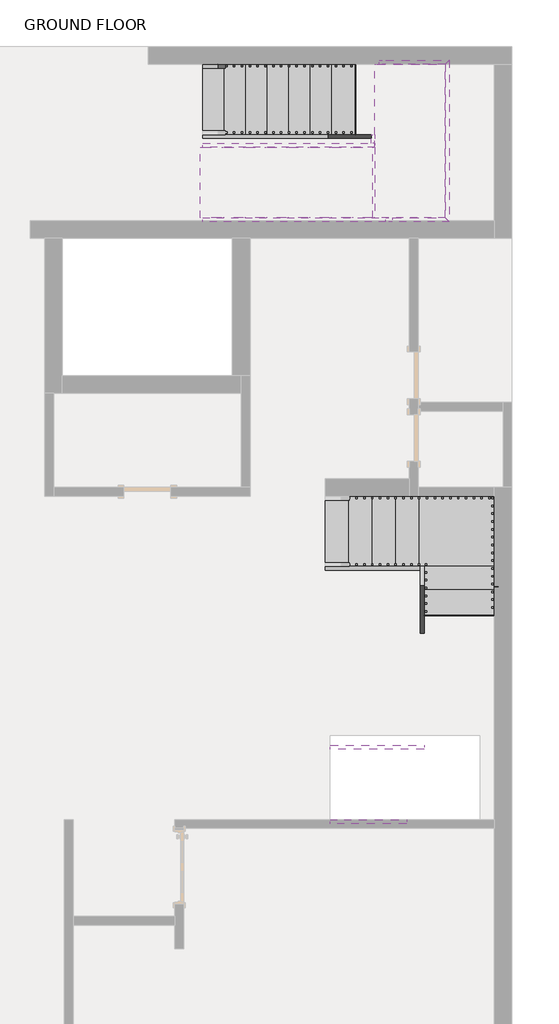
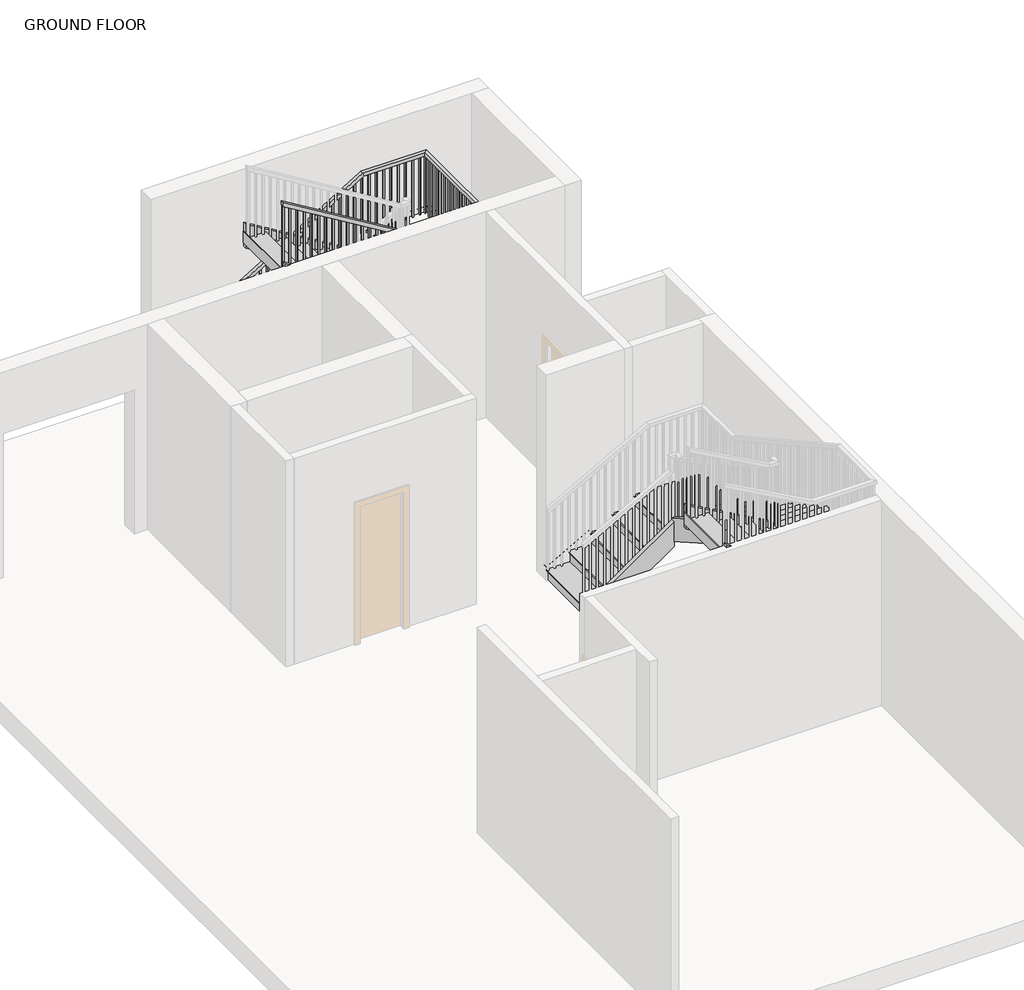
# One storey, part 3 of 3: 14 members, 3 stair flights, 1 railing, 1 slab.
"""IFC4 building model written with IfcOpenShell, lengths in millimetres."""

from ifc_helpers import new_model, si_unit, frame, origin, place, context, project, spatial, polyline, outline, extrude, faceted_brep, transform, mapped, element, save
from components import non_monolithic_landing_7100f040, stair_flight_950fb465, stair_flight_7c070f41, stair_flight_4d0103da

model = new_model("IFC4")

# Units and contexts
model_context = context("Model", 3, world=origin())
ifc_project = project(units=[si_unit("LENGTHUNIT", "METRE", prefix="MILLI")], contexts=[model_context])

# Site, building, storey
site = spatial("IfcSite", under=ifc_project)
building = spatial("IfcBuilding", under=site)
storey = spatial("IfcBuildingStorey", under=building, Name="GROUND FLOOR", Elevation=304.8)

# Members
placement = place(None, origin())
element("IfcMember", 1, ObjectType="Stringer - 2\" Width", at=placement, inside=storey, context=model_context, shape_type="SweptSolid", body=[
    extrude(outline(polyline([(516.914512, -12941.4571222), (304.8, -12941.4571222), (304.8, -12703.3716105), (1600.2, -10565.9616105), (1905.0, -10651.116067), (516.914512, -12941.4571222)])), frame((0.0, 7668.4964313, 0.0), z_axis=(0.0, 1.0, 0.0), x_axis=(0.0, 0.0, 1.0)), (0.0, 0.0, 1.0), 50.8),
])
element("IfcMember", 2, ObjectType="Stringer - 2\" Width", at=placement, inside=storey, context=model_context, shape_type="SweptSolid", body=[
    extrude(outline(polyline([(516.914512, -12941.4571222), (304.8, -12941.4571222), (304.8, -12703.3716105), (1484.3845383, -10757.0571222), (1840.7932998, -10757.0571222), (516.914512, -12941.4571222)])), frame((0.0, 6703.2964313, 0.0), z_axis=(0.0, 1.0, 0.0), x_axis=(0.0, 0.0, 1.0)), (0.0, 0.0, 1.0), 50.8),
])
element("IfcMember", 3, ObjectType="Stringer - 2\" Width", at=placement, inside=storey, context=model_context, shape_type="SweptSolid", body=[
    extrude(outline(polyline([(1600.2, -10567.152634), (1905.0, -10481.9981775), (3395.5811786, -12941.4571222), (3039.1724171, -12941.4571222), (1600.2, -10567.152634)])), frame((0.0, 5622.1776214, 0.0), z_axis=(0.0, 1.0, 0.0), x_axis=(0.0, 0.0, 1.0)), (0.0, 0.0, 1.0), 50.8),
])
element("IfcMember", 4, ObjectType="Stringer - 2\" Width", at=placement, inside=storey, context=model_context, shape_type="SweptSolid", body=[
    extrude(outline(polyline([(1684.5057504, -10706.2571222), (2040.914512, -10706.2571222), (3395.5811786, -12941.4571222), (3039.1724171, -12941.4571222), (1684.5057504, -10706.2571222)])), frame((0.0, 6587.3776214, 0.0), z_axis=(0.0, 1.0, 0.0), x_axis=(0.0, 0.0, 1.0)), (0.0, 0.0, 1.0), 50.8),
])
element("IfcMember", 5, ObjectType="Stringer - 2\" Width", at=placement, inside=storey, context=model_context, shape_type="Brep", body=[
    faceted_brep([(-10481.9981775, 5672.9776214, 1905.0), (-10481.9981775, 5622.1776214, 1905.0), (-9741.0571222, 5622.1776214, 1905.0), (-9791.8571222, 5672.9776214, 1905.0), (-10567.152634, 5672.9776214, 1600.2), (-9791.8571222, 5672.9776214, 1600.2), (-10567.152634, 5622.1776214, 1600.2), (-9741.0571222, 5622.1776214, 1600.2)], [[[0, 1, 2, 3]], [[4, 0, 3, 5]], [[6, 4, 5, 7]], [[1, 6, 7, 2]], [[1, 0, 4, 6]], [[2, 7, 5, 3]]]),
])
element("IfcMember", 6, ObjectType="Stringer - 2\" Width", at=placement, inside=storey, context=model_context, shape_type="SweptSolid", body=[
    extrude(outline(polyline([(-9741.0571222, 5622.1776214), (-9791.8571222, 5672.9776214), (-9791.8571222, 7668.4964313), (-9741.0571222, 7719.2964313), (-9741.0571222, 5622.1776214)])), frame((0.0, 0.0, 1600.2), z_axis=(0.0, 0.0, 1.0), x_axis=(1.0, 0.0, 0.0)), (0.0, 0.0, 1.0), 304.8),
])
element("IfcMember", 7, ObjectType="Stringer - 2\" Width", at=placement, inside=storey, context=model_context, shape_type="Brep", body=[
    faceted_brep([(-9791.8571222, 7668.4964313, 1905.0), (-9741.0571222, 7719.2964313, 1905.0), (-10651.116067, 7719.2964313, 1905.0), (-10651.116067, 7668.4964313, 1905.0), (-9791.8571222, 7668.4964313, 1600.2), (-10565.9616105, 7668.4964313, 1600.2), (-9741.0571222, 7719.2964313, 1600.2), (-10565.9616105, 7719.2964313, 1600.2)], [[[0, 1, 2, 3]], [[4, 0, 3, 5]], [[6, 4, 5, 7]], [[1, 6, 7, 2]], [[1, 0, 4, 6]], [[2, 7, 5, 3]]]),
])
element("IfcMember", 8, ObjectType="Stringer - 2\" Width", at=placement, inside=storey, context=model_context, shape_type="SweptSolid", body=[
    extrude(outline(polyline([(-10757.0571222, 6754.0964313), (-10706.2571222, 6754.0964313), (-10706.2571222, 6638.1776214), (-10757.0571222, 6638.1776214), (-10757.0571222, 6754.0964313)])), frame((0.0, 0.0, 1600.2), z_axis=(0.0, 0.0, 1.0), x_axis=(1.0, 0.0, 0.0)), (0.0, 0.0, 1.0), 304.8),
])
element("IfcMember", 9, ObjectType="Stringer - 2\" Width", at=placement, inside=storey, context=model_context, shape_type="SweptSolid", body=[
    extrude(outline(polyline([(512.3983948, -11350.6229553), (304.8, -11350.6229553), (304.8, -11096.6784525), (851.0650614, -10113.4013419), (851.0650614, -10741.0229553), (512.3983948, -11350.6229553)])), frame((0.0, 2055.0964313, 0.0), z_axis=(0.0, 1.0, 0.0), x_axis=(0.0, 0.0, 1.0)), (0.0, 0.0, 1.0), 50.8),
])
element("IfcMember", 10, ObjectType="Stringer - 2\" Width", at=placement, inside=storey, context=model_context, shape_type="SweptSolid", body=[
    extrude(outline(polyline([(467.5964313, 1384.3308318), (-1010.9251821, 2205.7317281), (-383.3035687, 2205.7317281), (1095.2180447, 1384.3308318), (467.5964313, 1384.3308318)])), frame((-9153.5229553, 0.0, 0.0), z_axis=(1.0, 0.0, 0.0), x_axis=(0.0, 1.0, 0.0)), (0.0, 0.0, 1.0), 50.8),
])
element("IfcMember", 11, ObjectType="Stringer - 2\" Width", at=placement, inside=storey, context=model_context, shape_type="SweptSolid", body=[
    extrude(outline(polyline([(2837.7752762, -10291.2013419), (3391.0650614, -11287.1229553), (3042.3863873, -11287.1229553), (2837.7752762, -10918.8229553), (2837.7752762, -10291.2013419)])), frame((0.0, -2199.4035687, 0.0), z_axis=(0.0, 1.0, 0.0), x_axis=(0.0, 0.0, 1.0)), (0.0, 0.0, 1.0), 50.8),
])
element("IfcMember", 12, ObjectType="Stringer - 2\" Width", at=placement, inside=storey, context=model_context, shape_type="SweptSolid", body=[
    extrude(outline(polyline([(483.7545455, -11350.6229553), (304.8, -11350.6229553), (304.8, -11073.6835803), (966.2445887, -10118.7229553), (1337.0186147, -10118.7229553), (483.7545455, -11350.6229553)])), frame((0.0, 1089.8964313, 0.0), z_axis=(0.0, 1.0, 0.0), x_axis=(0.0, 0.0, 1.0)), (0.0, 0.0, 1.0), 50.8),
])
element("IfcMember", 13, ObjectType="Stringer - 2\" Width", at=placement, inside=storey, context=model_context, shape_type="SweptSolid", body=[
    extrude(outline(polyline([(1140.6964313, 1360.35183), (1140.6964313, 1009.4520233), (-1183.4035687, 2335.1418629), (-1183.4035687, 2686.0416696), (1140.6964313, 1360.35183)])), frame((-10118.7229553, 0.0, 0.0), z_axis=(1.0, 0.0, 0.0), x_axis=(0.0, 1.0, 0.0)), (0.0, 0.0, 1.0), 50.8),
])
element("IfcMember", 14, ObjectType="Stringer - 2\" Width", at=placement, inside=storey, context=model_context, shape_type="SweptSolid", body=[
    extrude(outline(polyline([(2365.053054, -10067.9229553), (2713.7317281, -10067.9229553), (3391.0650614, -11287.1229553), (3042.3863873, -11287.1229553), (2365.053054, -10067.9229553)])), frame((0.0, -1234.2035687, 0.0), z_axis=(0.0, 1.0, 0.0), x_axis=(0.0, 0.0, 1.0)), (0.0, 0.0, 1.0), 50.8),
])

# Railing
element("IfcRailing", 15, ObjectType="Handrail - Rectangular", at=placement, inside=storey, context=model_context, shape_type="SolidModel", body=[
    faceted_brep([(-12941.4571222, 7668.4964313, 1388.5333333), (-12941.4571222, 7668.4964313, 1329.1318731), (-12941.4571222, 7617.6964313, 1329.1318731), (-12941.4571222, 7617.6964313, 1388.5333333), (-10706.2571222, 7668.4964313, 2743.2), (-10692.0647128, 7668.4964313, 2692.4), (-10692.0647128, 7617.6964313, 2692.4), (-10706.2571222, 7617.6964313, 2743.2), (-9791.8571222, 7668.4964313, 2743.2), (-9791.8571222, 7668.4964313, 2692.4), (-9842.6571222, 7617.6964313, 2692.4), (-9842.6571222, 7617.6964313, 2743.2), (-9791.8571222, 5672.9776214, 2743.2), (-9791.8571222, 5672.9776214, 2692.4), (-9842.6571222, 5723.7776214, 2692.4), (-9842.6571222, 5723.7776214, 2743.2), (-10426.8571222, 5672.9776214, 2743.2), (-10441.0495316, 5672.9776214, 2692.4), (-10441.0495316, 5723.7776214, 2692.4), (-10426.8571222, 5723.7776214, 2743.2), (-10706.2571222, 5672.9776214, 2912.5333333), (-10732.5868494, 5672.9776214, 2869.0892835), (-10732.5868494, 5723.7776214, 2869.0892835), (-10706.2571222, 5723.7776214, 2912.5333333), (-12941.4571222, 5672.9776214, 4267.2), (-12941.4571222, 5723.7776214, 4267.2), (-12941.4571222, 5723.7776214, 4207.7985397), (-12941.4571222, 5672.9776214, 4207.7985397)], [[[0, 1, 2, 3]], [[1, 0, 4, 5]], [[2, 1, 5, 6]], [[3, 2, 6, 7]], [[0, 3, 7, 4]], [[5, 4, 8, 9]], [[6, 5, 9, 10]], [[7, 6, 10, 11]], [[4, 7, 11, 8]], [[9, 8, 12, 13]], [[10, 9, 13, 14]], [[11, 10, 14, 15]], [[8, 11, 15, 12]], [[13, 12, 16, 17]], [[14, 13, 17, 18]], [[15, 14, 18, 19]], [[12, 15, 19, 16]], [[17, 16, 20, 21]], [[18, 17, 21, 22]], [[19, 18, 22, 23]], [[16, 19, 23, 20]], [[24, 25, 26, 27]], [[21, 20, 24, 27]], [[22, 21, 27, 26]], [[23, 22, 26, 25]], [[20, 23, 25, 24]]]),
    extrude(outline(polyline([(4151.9955094, -12849.3821222), (3183.4666667, -12849.3821222), (3183.4666667, -12830.3321222), (4140.4500549, -12830.3321222), (4151.9955094, -12849.3821222)])), frame((0.0, 5688.8526214, 0.0), z_axis=(0.0, 1.0, 0.0), x_axis=(0.0, 0.0, 1.0)), (0.0, 0.0, 1.0), 19.05),
    extrude(outline(polyline([(4090.4197519, -12747.7821222), (3183.4666667, -12747.7821222), (3183.4666667, -12728.7321222), (4078.8742973, -12728.7321222), (4090.4197519, -12747.7821222)])), frame((0.0, 5688.8526214, 0.0), z_axis=(0.0, 1.0, 0.0), x_axis=(0.0, 0.0, 1.0)), (0.0, 0.0, 1.0), 19.05),
    extrude(outline(polyline([(4028.8439943, -12646.1821222), (3014.1333333, -12646.1821222), (3014.1333333, -12627.1321222), (4017.2985397, -12627.1321222), (4028.8439943, -12646.1821222)])), frame((0.0, 5688.8526214, 0.0), z_axis=(0.0, 1.0, 0.0), x_axis=(0.0, 0.0, 1.0)), (0.0, 0.0, 1.0), 19.05),
    extrude(outline(polyline([(3967.2682367, -12544.5821222), (3014.1333333, -12544.5821222), (3014.1333333, -12525.5321222), (3955.7227822, -12525.5321222), (3967.2682367, -12544.5821222)])), frame((0.0, 5688.8526214, 0.0), z_axis=(0.0, 1.0, 0.0), x_axis=(0.0, 0.0, 1.0)), (0.0, 0.0, 1.0), 19.05),
    extrude(outline(polyline([(3905.6924791, -12442.9821222), (3014.1333333, -12442.9821222), (3014.1333333, -12423.9321222), (3894.1470246, -12423.9321222), (3905.6924791, -12442.9821222)])), frame((0.0, 5688.8526214, 0.0), z_axis=(0.0, 1.0, 0.0), x_axis=(0.0, 0.0, 1.0)), (0.0, 0.0, 1.0), 19.05),
    extrude(outline(polyline([(3844.1167216, -12341.3821222), (2844.8, -12341.3821222), (2844.8, -12322.3321222), (3832.571267, -12322.3321222), (3844.1167216, -12341.3821222)])), frame((0.0, 5688.8526214, 0.0), z_axis=(0.0, 1.0, 0.0), x_axis=(0.0, 0.0, 1.0)), (0.0, 0.0, 1.0), 19.05),
    extrude(outline(polyline([(3782.540964, -12239.7821222), (2844.8, -12239.7821222), (2844.8, -12220.7321222), (3770.9955094, -12220.7321222), (3782.540964, -12239.7821222)])), frame((0.0, 5688.8526214, 0.0), z_axis=(0.0, 1.0, 0.0), x_axis=(0.0, 0.0, 1.0)), (0.0, 0.0, 1.0), 19.05),
    extrude(outline(polyline([(3720.9652064, -12138.1821222), (2844.8, -12138.1821222), (2844.8, -12119.1321222), (3709.4197519, -12119.1321222), (3720.9652064, -12138.1821222)])), frame((0.0, 5688.8526214, 0.0), z_axis=(0.0, 1.0, 0.0), x_axis=(0.0, 0.0, 1.0)), (0.0, 0.0, 1.0), 19.05),
    extrude(outline(polyline([(3659.3894488, -12036.5821222), (2675.4666667, -12036.5821222), (2675.4666667, -12017.5321222), (3647.8439943, -12017.5321222), (3659.3894488, -12036.5821222)])), frame((0.0, 5688.8526214, 0.0), z_axis=(0.0, 1.0, 0.0), x_axis=(0.0, 0.0, 1.0)), (0.0, 0.0, 1.0), 19.05),
    extrude(outline(polyline([(3597.8136913, -11934.9821222), (2675.4666667, -11934.9821222), (2675.4666667, -11915.9321222), (3586.2682367, -11915.9321222), (3597.8136913, -11934.9821222)])), frame((0.0, 5688.8526214, 0.0), z_axis=(0.0, 1.0, 0.0), x_axis=(0.0, 0.0, 1.0)), (0.0, 0.0, 1.0), 19.05),
    extrude(outline(polyline([(3536.2379337, -11833.3821222), (2675.4666667, -11833.3821222), (2675.4666667, -11814.3321222), (3524.6924791, -11814.3321222), (3536.2379337, -11833.3821222)])), frame((0.0, 5688.8526214, 0.0), z_axis=(0.0, 1.0, 0.0), x_axis=(0.0, 0.0, 1.0)), (0.0, 0.0, 1.0), 19.05),
    extrude(outline(polyline([(3474.6621761, -11731.7821222), (2506.1333333, -11731.7821222), (2506.1333333, -11712.7321222), (3463.1167216, -11712.7321222), (3474.6621761, -11731.7821222)])), frame((0.0, 5688.8526214, 0.0), z_axis=(0.0, 1.0, 0.0), x_axis=(0.0, 0.0, 1.0)), (0.0, 0.0, 1.0), 19.05),
    extrude(outline(polyline([(3413.0864185, -11630.1821222), (2506.1333333, -11630.1821222), (2506.1333333, -11611.1321222), (3401.540964, -11611.1321222), (3413.0864185, -11630.1821222)])), frame((0.0, 5688.8526214, 0.0), z_axis=(0.0, 1.0, 0.0), x_axis=(0.0, 0.0, 1.0)), (0.0, 0.0, 1.0), 19.05),
    extrude(outline(polyline([(3351.510661, -11528.5821222), (2336.8, -11528.5821222), (2336.8, -11509.5321222), (3339.9652064, -11509.5321222), (3351.510661, -11528.5821222)])), frame((0.0, 5688.8526214, 0.0), z_axis=(0.0, 1.0, 0.0), x_axis=(0.0, 0.0, 1.0)), (0.0, 0.0, 1.0), 19.05),
    extrude(outline(polyline([(3289.9349034, -11426.9821222), (2336.8, -11426.9821222), (2336.8, -11407.9321222), (3278.3894488, -11407.9321222), (3289.9349034, -11426.9821222)])), frame((0.0, 5688.8526214, 0.0), z_axis=(0.0, 1.0, 0.0), x_axis=(0.0, 0.0, 1.0)), (0.0, 0.0, 1.0), 19.05),
    extrude(outline(polyline([(3228.3591458, -11325.3821222), (2336.8, -11325.3821222), (2336.8, -11306.3321222), (3216.8136913, -11306.3321222), (3228.3591458, -11325.3821222)])), frame((0.0, 5688.8526214, 0.0), z_axis=(0.0, 1.0, 0.0), x_axis=(0.0, 0.0, 1.0)), (0.0, 0.0, 1.0), 19.05),
    extrude(outline(polyline([(3166.7833882, -11223.7821222), (2167.4666667, -11223.7821222), (2167.4666667, -11204.7321222), (3155.2379337, -11204.7321222), (3166.7833882, -11223.7821222)])), frame((0.0, 5688.8526214, 0.0), z_axis=(0.0, 1.0, 0.0), x_axis=(0.0, 0.0, 1.0)), (0.0, 0.0, 1.0), 19.05),
    extrude(outline(polyline([(3105.2076307, -11122.1821222), (2167.4666667, -11122.1821222), (2167.4666667, -11103.1321222), (3093.6621761, -11103.1321222), (3105.2076307, -11122.1821222)])), frame((0.0, 5688.8526214, 0.0), z_axis=(0.0, 1.0, 0.0), x_axis=(0.0, 0.0, 1.0)), (0.0, 0.0, 1.0), 19.05),
    extrude(outline(polyline([(3043.6318731, -11020.5821222), (2167.4666667, -11020.5821222), (2167.4666667, -11001.5321222), (3032.0864185, -11001.5321222), (3043.6318731, -11020.5821222)])), frame((0.0, 5688.8526214, 0.0), z_axis=(0.0, 1.0, 0.0), x_axis=(0.0, 0.0, 1.0)), (0.0, 0.0, 1.0), 19.05),
    extrude(outline(polyline([(2982.0561155, -10918.9821222), (1998.1333333, -10918.9821222), (1998.1333333, -10899.9321222), (2970.510661, -10899.9321222), (2982.0561155, -10918.9821222)])), frame((0.0, 5688.8526214, 0.0), z_axis=(0.0, 1.0, 0.0), x_axis=(0.0, 0.0, 1.0)), (0.0, 0.0, 1.0), 19.05),
    extrude(outline(polyline([(2920.4803579, -10817.3821222), (1998.1333333, -10817.3821222), (1998.1333333, -10798.3321222), (2908.9349034, -10798.3321222), (2920.4803579, -10817.3821222)])), frame((0.0, 5688.8526214, 0.0), z_axis=(0.0, 1.0, 0.0), x_axis=(0.0, 0.0, 1.0)), (0.0, 0.0, 1.0), 19.05),
    extrude(outline(polyline([(2812.7227822, -10639.5821222), (1828.8, -10639.5821222), (1828.8, -10620.5321222), (2801.1773276, -10620.5321222), (2812.7227822, -10639.5821222)])), frame((0.0, 5688.8526214, 0.0), z_axis=(0.0, 1.0, 0.0), x_axis=(0.0, 0.0, 1.0)), (0.0, 0.0, 1.0), 19.05),
    extrude(outline(polyline([(2751.1470246, -10537.9821222), (1828.8, -10537.9821222), (1828.8, -10518.9321222), (2739.60157, -10518.9321222), (2751.1470246, -10537.9821222)])), frame((0.0, 5688.8526214, 0.0), z_axis=(0.0, 1.0, 0.0), x_axis=(0.0, 0.0, 1.0)), (0.0, 0.0, 1.0), 19.05),
    extrude(outline(polyline([(-10417.3321222, 5688.8526214), (-10436.3821222, 5688.8526214), (-10436.3821222, 5707.9026214), (-10417.3321222, 5707.9026214), (-10417.3321222, 5688.8526214)])), frame((0.0, 0.0, 1828.8), z_axis=(0.0, 0.0, 1.0), x_axis=(1.0, 0.0, 0.0)), (0.0, 0.0, 1.0), 863.6),
    extrude(outline(polyline([(-10315.7321222, 5688.8526214), (-10334.7821222, 5688.8526214), (-10334.7821222, 5707.9026214), (-10315.7321222, 5707.9026214), (-10315.7321222, 5688.8526214)])), frame((0.0, 0.0, 1828.8), z_axis=(0.0, 0.0, 1.0), x_axis=(1.0, 0.0, 0.0)), (0.0, 0.0, 1.0), 863.6),
    extrude(outline(polyline([(-10214.1321222, 5688.8526214), (-10233.1821222, 5688.8526214), (-10233.1821222, 5707.9026214), (-10214.1321222, 5707.9026214), (-10214.1321222, 5688.8526214)])), frame((0.0, 0.0, 1828.8), z_axis=(0.0, 0.0, 1.0), x_axis=(1.0, 0.0, 0.0)), (0.0, 0.0, 1.0), 863.6),
    extrude(outline(polyline([(-10112.5321222, 5688.8526214), (-10131.5821222, 5688.8526214), (-10131.5821222, 5707.9026214), (-10112.5321222, 5707.9026214), (-10112.5321222, 5688.8526214)])), frame((0.0, 0.0, 1828.8), z_axis=(0.0, 0.0, 1.0), x_axis=(1.0, 0.0, 0.0)), (0.0, 0.0, 1.0), 863.6),
    extrude(outline(polyline([(-10010.9321222, 5688.8526214), (-10029.9821222, 5688.8526214), (-10029.9821222, 5707.9026214), (-10010.9321222, 5707.9026214), (-10010.9321222, 5688.8526214)])), frame((0.0, 0.0, 1828.8), z_axis=(0.0, 0.0, 1.0), x_axis=(1.0, 0.0, 0.0)), (0.0, 0.0, 1.0), 863.6),
    extrude(outline(polyline([(-9909.3321222, 5688.8526214), (-9928.3821222, 5688.8526214), (-9928.3821222, 5707.9026214), (-9909.3321222, 5707.9026214), (-9909.3321222, 5688.8526214)])), frame((0.0, 0.0, 1828.8), z_axis=(0.0, 0.0, 1.0), x_axis=(1.0, 0.0, 0.0)), (0.0, 0.0, 1.0), 863.6),
    extrude(outline(polyline([(-9807.7321222, 5722.2214313), (-9807.7321222, 5703.1714313), (-9826.7821222, 5703.1714313), (-9826.7821222, 5722.2214313), (-9807.7321222, 5722.2214313)])), frame((0.0, 0.0, 1828.8), z_axis=(0.0, 0.0, 1.0), x_axis=(1.0, 0.0, 0.0)), (0.0, 0.0, 1.0), 863.6),
    extrude(outline(polyline([(-9807.7321222, 5823.8214313), (-9807.7321222, 5804.7714313), (-9826.7821222, 5804.7714313), (-9826.7821222, 5823.8214313), (-9807.7321222, 5823.8214313)])), frame((0.0, 0.0, 1828.8), z_axis=(0.0, 0.0, 1.0), x_axis=(1.0, 0.0, 0.0)), (0.0, 0.0, 1.0), 863.6),
    extrude(outline(polyline([(-9807.7321222, 5925.4214313), (-9807.7321222, 5906.3714313), (-9826.7821222, 5906.3714313), (-9826.7821222, 5925.4214313), (-9807.7321222, 5925.4214313)])), frame((0.0, 0.0, 1828.8), z_axis=(0.0, 0.0, 1.0), x_axis=(1.0, 0.0, 0.0)), (0.0, 0.0, 1.0), 863.6),
    extrude(outline(polyline([(-9807.7321222, 6027.0214313), (-9807.7321222, 6007.9714313), (-9826.7821222, 6007.9714313), (-9826.7821222, 6027.0214313), (-9807.7321222, 6027.0214313)])), frame((0.0, 0.0, 1828.8), z_axis=(0.0, 0.0, 1.0), x_axis=(1.0, 0.0, 0.0)), (0.0, 0.0, 1.0), 863.6),
    extrude(outline(polyline([(-9807.7321222, 6128.6214313), (-9807.7321222, 6109.5714313), (-9826.7821222, 6109.5714313), (-9826.7821222, 6128.6214313), (-9807.7321222, 6128.6214313)])), frame((0.0, 0.0, 1828.8), z_axis=(0.0, 0.0, 1.0), x_axis=(1.0, 0.0, 0.0)), (0.0, 0.0, 1.0), 863.6),
    extrude(outline(polyline([(-9807.7321222, 6230.2214313), (-9807.7321222, 6211.1714313), (-9826.7821222, 6211.1714313), (-9826.7821222, 6230.2214313), (-9807.7321222, 6230.2214313)])), frame((0.0, 0.0, 1828.8), z_axis=(0.0, 0.0, 1.0), x_axis=(1.0, 0.0, 0.0)), (0.0, 0.0, 1.0), 863.6),
    extrude(outline(polyline([(-9807.7321222, 6331.8214313), (-9807.7321222, 6312.7714313), (-9826.7821222, 6312.7714313), (-9826.7821222, 6331.8214313), (-9807.7321222, 6331.8214313)])), frame((0.0, 0.0, 1828.8), z_axis=(0.0, 0.0, 1.0), x_axis=(1.0, 0.0, 0.0)), (0.0, 0.0, 1.0), 863.6),
    extrude(outline(polyline([(-9807.7321222, 6433.4214313), (-9807.7321222, 6414.3714313), (-9826.7821222, 6414.3714313), (-9826.7821222, 6433.4214313), (-9807.7321222, 6433.4214313)])), frame((0.0, 0.0, 1828.8), z_axis=(0.0, 0.0, 1.0), x_axis=(1.0, 0.0, 0.0)), (0.0, 0.0, 1.0), 863.6),
    extrude(outline(polyline([(-9807.7321222, 6535.0214313), (-9807.7321222, 6515.9714313), (-9826.7821222, 6515.9714313), (-9826.7821222, 6535.0214313), (-9807.7321222, 6535.0214313)])), frame((0.0, 0.0, 1828.8), z_axis=(0.0, 0.0, 1.0), x_axis=(1.0, 0.0, 0.0)), (0.0, 0.0, 1.0), 863.6),
    extrude(outline(polyline([(-9807.7321222, 6636.6214313), (-9807.7321222, 6617.5714313), (-9826.7821222, 6617.5714313), (-9826.7821222, 6636.6214313), (-9807.7321222, 6636.6214313)])), frame((0.0, 0.0, 1828.8), z_axis=(0.0, 0.0, 1.0), x_axis=(1.0, 0.0, 0.0)), (0.0, 0.0, 1.0), 863.6),
    extrude(outline(polyline([(-9807.7321222, 6738.2214313), (-9807.7321222, 6719.1714313), (-9826.7821222, 6719.1714313), (-9826.7821222, 6738.2214313), (-9807.7321222, 6738.2214313)])), frame((0.0, 0.0, 1828.8), z_axis=(0.0, 0.0, 1.0), x_axis=(1.0, 0.0, 0.0)), (0.0, 0.0, 1.0), 863.6),
    extrude(outline(polyline([(-9807.7321222, 6839.8214313), (-9807.7321222, 6820.7714313), (-9826.7821222, 6820.7714313), (-9826.7821222, 6839.8214313), (-9807.7321222, 6839.8214313)])), frame((0.0, 0.0, 1828.8), z_axis=(0.0, 0.0, 1.0), x_axis=(1.0, 0.0, 0.0)), (0.0, 0.0, 1.0), 863.6),
    extrude(outline(polyline([(-9807.7321222, 6941.4214313), (-9807.7321222, 6922.3714313), (-9826.7821222, 6922.3714313), (-9826.7821222, 6941.4214313), (-9807.7321222, 6941.4214313)])), frame((0.0, 0.0, 1828.8), z_axis=(0.0, 0.0, 1.0), x_axis=(1.0, 0.0, 0.0)), (0.0, 0.0, 1.0), 863.6),
    extrude(outline(polyline([(-9807.7321222, 7043.0214313), (-9807.7321222, 7023.9714313), (-9826.7821222, 7023.9714313), (-9826.7821222, 7043.0214313), (-9807.7321222, 7043.0214313)])), frame((0.0, 0.0, 1828.8), z_axis=(0.0, 0.0, 1.0), x_axis=(1.0, 0.0, 0.0)), (0.0, 0.0, 1.0), 863.6),
    extrude(outline(polyline([(-9807.7321222, 7144.6214313), (-9807.7321222, 7125.5714313), (-9826.7821222, 7125.5714313), (-9826.7821222, 7144.6214313), (-9807.7321222, 7144.6214313)])), frame((0.0, 0.0, 1828.8), z_axis=(0.0, 0.0, 1.0), x_axis=(1.0, 0.0, 0.0)), (0.0, 0.0, 1.0), 863.6),
    extrude(outline(polyline([(-9807.7321222, 7246.2214313), (-9807.7321222, 7227.1714313), (-9826.7821222, 7227.1714313), (-9826.7821222, 7246.2214313), (-9807.7321222, 7246.2214313)])), frame((0.0, 0.0, 1828.8), z_axis=(0.0, 0.0, 1.0), x_axis=(1.0, 0.0, 0.0)), (0.0, 0.0, 1.0), 863.6),
    extrude(outline(polyline([(-9807.7321222, 7347.8214313), (-9807.7321222, 7328.7714313), (-9826.7821222, 7328.7714313), (-9826.7821222, 7347.8214313), (-9807.7321222, 7347.8214313)])), frame((0.0, 0.0, 1828.8), z_axis=(0.0, 0.0, 1.0), x_axis=(1.0, 0.0, 0.0)), (0.0, 0.0, 1.0), 863.6),
    extrude(outline(polyline([(-9807.7321222, 7449.4214313), (-9807.7321222, 7430.3714313), (-9826.7821222, 7430.3714313), (-9826.7821222, 7449.4214313), (-9807.7321222, 7449.4214313)])), frame((0.0, 0.0, 1828.8), z_axis=(0.0, 0.0, 1.0), x_axis=(1.0, 0.0, 0.0)), (0.0, 0.0, 1.0), 863.6),
    extrude(outline(polyline([(-9807.7321222, 7551.0214313), (-9807.7321222, 7531.9714313), (-9826.7821222, 7531.9714313), (-9826.7821222, 7551.0214313), (-9807.7321222, 7551.0214313)])), frame((0.0, 0.0, 1828.8), z_axis=(0.0, 0.0, 1.0), x_axis=(1.0, 0.0, 0.0)), (0.0, 0.0, 1.0), 863.6),
    extrude(outline(polyline([(-9902.9821222, 7652.6214313), (-9883.9321222, 7652.6214313), (-9883.9321222, 7633.5714313), (-9902.9821222, 7633.5714313), (-9902.9821222, 7652.6214313)])), frame((0.0, 0.0, 1828.8), z_axis=(0.0, 0.0, 1.0), x_axis=(1.0, 0.0, 0.0)), (0.0, 0.0, 1.0), 863.6),
    extrude(outline(polyline([(-10004.5821222, 7652.6214313), (-9985.5321222, 7652.6214313), (-9985.5321222, 7633.5714313), (-10004.5821222, 7633.5714313), (-10004.5821222, 7652.6214313)])), frame((0.0, 0.0, 1828.8), z_axis=(0.0, 0.0, 1.0), x_axis=(1.0, 0.0, 0.0)), (0.0, 0.0, 1.0), 863.6),
    extrude(outline(polyline([(-10106.1821222, 7652.6214313), (-10087.1321222, 7652.6214313), (-10087.1321222, 7633.5714313), (-10106.1821222, 7633.5714313), (-10106.1821222, 7652.6214313)])), frame((0.0, 0.0, 1828.8), z_axis=(0.0, 0.0, 1.0), x_axis=(1.0, 0.0, 0.0)), (0.0, 0.0, 1.0), 863.6),
    extrude(outline(polyline([(-10207.7821222, 7652.6214313), (-10188.7321222, 7652.6214313), (-10188.7321222, 7633.5714313), (-10207.7821222, 7633.5714313), (-10207.7821222, 7652.6214313)])), frame((0.0, 0.0, 1828.8), z_axis=(0.0, 0.0, 1.0), x_axis=(1.0, 0.0, 0.0)), (0.0, 0.0, 1.0), 863.6),
    extrude(outline(polyline([(-10309.3821222, 7652.6214313), (-10290.3321222, 7652.6214313), (-10290.3321222, 7633.5714313), (-10309.3821222, 7633.5714313), (-10309.3821222, 7652.6214313)])), frame((0.0, 0.0, 1828.8), z_axis=(0.0, 0.0, 1.0), x_axis=(1.0, 0.0, 0.0)), (0.0, 0.0, 1.0), 863.6),
    extrude(outline(polyline([(-10410.9821222, 7652.6214313), (-10391.9321222, 7652.6214313), (-10391.9321222, 7633.5714313), (-10410.9821222, 7633.5714313), (-10410.9821222, 7652.6214313)])), frame((0.0, 0.0, 1828.8), z_axis=(0.0, 0.0, 1.0), x_axis=(1.0, 0.0, 0.0)), (0.0, 0.0, 1.0), 863.6),
    extrude(outline(polyline([(-10512.5821222, 7652.6214313), (-10493.5321222, 7652.6214313), (-10493.5321222, 7633.5714313), (-10512.5821222, 7633.5714313), (-10512.5821222, 7652.6214313)])), frame((0.0, 0.0, 1828.8), z_axis=(0.0, 0.0, 1.0), x_axis=(1.0, 0.0, 0.0)), (0.0, 0.0, 1.0), 863.6),
    extrude(outline(polyline([(-10614.1821222, 7652.6214313), (-10595.1321222, 7652.6214313), (-10595.1321222, 7633.5714313), (-10614.1821222, 7633.5714313), (-10614.1821222, 7652.6214313)])), frame((0.0, 0.0, 1828.8), z_axis=(0.0, 0.0, 1.0), x_axis=(1.0, 0.0, 0.0)), (0.0, 0.0, 1.0), 863.6),
    extrude(outline(polyline([(2616.4500549, -10817.3821222), (1659.4666667, -10817.3821222), (1659.4666667, -10798.3321222), (2627.9955094, -10798.3321222), (2616.4500549, -10817.3821222)])), frame((0.0, 7633.5714313, 0.0), z_axis=(0.0, 1.0, 0.0), x_axis=(0.0, 0.0, 1.0)), (0.0, 0.0, 1.0), 19.05),
    extrude(outline(polyline([(2554.8742973, -10918.9821222), (1659.4666667, -10918.9821222), (1659.4666667, -10899.9321222), (2566.4197519, -10899.9321222), (2554.8742973, -10918.9821222)])), frame((0.0, 7633.5714313, 0.0), z_axis=(0.0, 1.0, 0.0), x_axis=(0.0, 0.0, 1.0)), (0.0, 0.0, 1.0), 19.05),
    extrude(outline(polyline([(2493.2985397, -11020.5821222), (1490.1333333, -11020.5821222), (1490.1333333, -11001.5321222), (2504.8439943, -11001.5321222), (2493.2985397, -11020.5821222)])), frame((0.0, 7633.5714313, 0.0), z_axis=(0.0, 1.0, 0.0), x_axis=(0.0, 0.0, 1.0)), (0.0, 0.0, 1.0), 19.05),
    extrude(outline(polyline([(2431.7227822, -11122.1821222), (1490.1333333, -11122.1821222), (1490.1333333, -11103.1321222), (2443.2682367, -11103.1321222), (2431.7227822, -11122.1821222)])), frame((0.0, 7633.5714313, 0.0), z_axis=(0.0, 1.0, 0.0), x_axis=(0.0, 0.0, 1.0)), (0.0, 0.0, 1.0), 19.05),
    extrude(outline(polyline([(2370.1470246, -11223.7821222), (1490.1333333, -11223.7821222), (1490.1333333, -11204.7321222), (2381.6924791, -11204.7321222), (2370.1470246, -11223.7821222)])), frame((0.0, 7633.5714313, 0.0), z_axis=(0.0, 1.0, 0.0), x_axis=(0.0, 0.0, 1.0)), (0.0, 0.0, 1.0), 19.05),
    extrude(outline(polyline([(2308.571267, -11325.3821222), (1320.8, -11325.3821222), (1320.8, -11306.3321222), (2320.1167216, -11306.3321222), (2308.571267, -11325.3821222)])), frame((0.0, 7633.5714313, 0.0), z_axis=(0.0, 1.0, 0.0), x_axis=(0.0, 0.0, 1.0)), (0.0, 0.0, 1.0), 19.05),
    extrude(outline(polyline([(2246.9955094, -11426.9821222), (1320.8, -11426.9821222), (1320.8, -11407.9321222), (2258.540964, -11407.9321222), (2246.9955094, -11426.9821222)])), frame((0.0, 7633.5714313, 0.0), z_axis=(0.0, 1.0, 0.0), x_axis=(0.0, 0.0, 1.0)), (0.0, 0.0, 1.0), 19.05),
    extrude(outline(polyline([(2185.4197519, -11528.5821222), (1320.8, -11528.5821222), (1320.8, -11509.5321222), (2196.9652064, -11509.5321222), (2185.4197519, -11528.5821222)])), frame((0.0, 7633.5714313, 0.0), z_axis=(0.0, 1.0, 0.0), x_axis=(0.0, 0.0, 1.0)), (0.0, 0.0, 1.0), 19.05),
    extrude(outline(polyline([(2123.8439943, -11630.1821222), (1151.4666667, -11630.1821222), (1151.4666667, -11611.1321222), (2135.3894488, -11611.1321222), (2123.8439943, -11630.1821222)])), frame((0.0, 7633.5714313, 0.0), z_axis=(0.0, 1.0, 0.0), x_axis=(0.0, 0.0, 1.0)), (0.0, 0.0, 1.0), 19.05),
    extrude(outline(polyline([(2062.2682367, -11731.7821222), (1151.4666667, -11731.7821222), (1151.4666667, -11712.7321222), (2073.8136913, -11712.7321222), (2062.2682367, -11731.7821222)])), frame((0.0, 7633.5714313, 0.0), z_axis=(0.0, 1.0, 0.0), x_axis=(0.0, 0.0, 1.0)), (0.0, 0.0, 1.0), 19.05),
    extrude(outline(polyline([(2000.6924791, -11833.3821222), (1151.4666667, -11833.3821222), (1151.4666667, -11814.3321222), (2012.2379337, -11814.3321222), (2000.6924791, -11833.3821222)])), frame((0.0, 7633.5714313, 0.0), z_axis=(0.0, 1.0, 0.0), x_axis=(0.0, 0.0, 1.0)), (0.0, 0.0, 1.0), 19.05),
    extrude(outline(polyline([(1939.1167216, -11934.9821222), (982.1333333, -11934.9821222), (982.1333333, -11915.9321222), (1950.6621761, -11915.9321222), (1939.1167216, -11934.9821222)])), frame((0.0, 7633.5714313, 0.0), z_axis=(0.0, 1.0, 0.0), x_axis=(0.0, 0.0, 1.0)), (0.0, 0.0, 1.0), 19.05),
    extrude(outline(polyline([(1877.540964, -12036.5821222), (982.1333333, -12036.5821222), (982.1333333, -12017.5321222), (1889.0864185, -12017.5321222), (1877.540964, -12036.5821222)])), frame((0.0, 7633.5714313, 0.0), z_axis=(0.0, 1.0, 0.0), x_axis=(0.0, 0.0, 1.0)), (0.0, 0.0, 1.0), 19.05),
    extrude(outline(polyline([(1815.9652064, -12138.1821222), (812.8, -12138.1821222), (812.8, -12119.1321222), (1827.510661, -12119.1321222), (1815.9652064, -12138.1821222)])), frame((0.0, 7633.5714313, 0.0), z_axis=(0.0, 1.0, 0.0), x_axis=(0.0, 0.0, 1.0)), (0.0, 0.0, 1.0), 19.05),
    extrude(outline(polyline([(1754.3894488, -12239.7821222), (812.8, -12239.7821222), (812.8, -12220.7321222), (1765.9349034, -12220.7321222), (1754.3894488, -12239.7821222)])), frame((0.0, 7633.5714313, 0.0), z_axis=(0.0, 1.0, 0.0), x_axis=(0.0, 0.0, 1.0)), (0.0, 0.0, 1.0), 19.05),
    extrude(outline(polyline([(1692.8136913, -12341.3821222), (812.8, -12341.3821222), (812.8, -12322.3321222), (1704.3591458, -12322.3321222), (1692.8136913, -12341.3821222)])), frame((0.0, 7633.5714313, 0.0), z_axis=(0.0, 1.0, 0.0), x_axis=(0.0, 0.0, 1.0)), (0.0, 0.0, 1.0), 19.05),
    extrude(outline(polyline([(1631.2379337, -12442.9821222), (643.4666667, -12442.9821222), (643.4666667, -12423.9321222), (1642.7833882, -12423.9321222), (1631.2379337, -12442.9821222)])), frame((0.0, 7633.5714313, 0.0), z_axis=(0.0, 1.0, 0.0), x_axis=(0.0, 0.0, 1.0)), (0.0, 0.0, 1.0), 19.05),
    extrude(outline(polyline([(1569.6621761, -12544.5821222), (643.4666667, -12544.5821222), (643.4666667, -12525.5321222), (1581.2076307, -12525.5321222), (1569.6621761, -12544.5821222)])), frame((0.0, 7633.5714313, 0.0), z_axis=(0.0, 1.0, 0.0), x_axis=(0.0, 0.0, 1.0)), (0.0, 0.0, 1.0), 19.05),
    extrude(outline(polyline([(1508.0864185, -12646.1821222), (643.4666667, -12646.1821222), (643.4666667, -12627.1321222), (1519.6318731, -12627.1321222), (1508.0864185, -12646.1821222)])), frame((0.0, 7633.5714313, 0.0), z_axis=(0.0, 1.0, 0.0), x_axis=(0.0, 0.0, 1.0)), (0.0, 0.0, 1.0), 19.05),
    extrude(outline(polyline([(1446.510661, -12747.7821222), (474.1333333, -12747.7821222), (474.1333333, -12728.7321222), (1458.0561155, -12728.7321222), (1446.510661, -12747.7821222)])), frame((0.0, 7633.5714313, 0.0), z_axis=(0.0, 1.0, 0.0), x_axis=(0.0, 0.0, 1.0)), (0.0, 0.0, 1.0), 19.05),
    extrude(outline(polyline([(1384.9349034, -12849.3821222), (474.1333333, -12849.3821222), (474.1333333, -12830.3321222), (1396.4803579, -12830.3321222), (1384.9349034, -12849.3821222)])), frame((0.0, 7633.5714313, 0.0), z_axis=(0.0, 1.0, 0.0), x_axis=(0.0, 0.0, 1.0)), (0.0, 0.0, 1.0), 19.05),
    extrude(outline(polyline([(2858.9046004, -10715.7821222), (1828.8, -10715.7821222), (1828.8, -10696.7321222), (2847.3591458, -10696.7321222), (2858.9046004, -10715.7821222)])), frame((0.0, 5688.8526214, 0.0), z_axis=(0.0, 1.0, 0.0), x_axis=(0.0, 0.0, 1.0)), (0.0, 0.0, 1.0), 19.05),
    extrude(outline(polyline([(-9807.7321222, 5707.9026214), (-9807.7321222, 5688.8526214), (-9826.7821222, 5688.8526214), (-9826.7821222, 5707.9026214), (-9807.7321222, 5707.9026214)])), frame((0.0, 0.0, 1828.8), z_axis=(0.0, 0.0, 1.0), x_axis=(1.0, 0.0, 0.0)), (0.0, 0.0, 1.0), 863.6),
    extrude(outline(polyline([(-9826.7821222, 7652.6214313), (-9807.7321222, 7652.6214313), (-9807.7321222, 7633.5714313), (-9826.7821222, 7633.5714313), (-9826.7821222, 7652.6214313)])), frame((0.0, 0.0, 1828.8), z_axis=(0.0, 0.0, 1.0), x_axis=(1.0, 0.0, 0.0)), (0.0, 0.0, 1.0), 863.6),
    extrude(outline(polyline([(2678.0258125, -10715.7821222), (1828.8, -10715.7821222), (1828.8, -10696.7321222), (2689.571267, -10696.7321222), (2678.0258125, -10715.7821222)])), frame((0.0, 7633.5714313, 0.0), z_axis=(0.0, 1.0, 0.0), x_axis=(0.0, 0.0, 1.0)), (0.0, 0.0, 1.0), 19.05),
    extrude(outline(polyline([(4207.7985397, -12941.4571222), (3183.4666667, -12941.4571222), (3183.4666667, -12922.4071222), (4196.2530852, -12922.4071222), (4207.7985397, -12941.4571222)])), frame((0.0, 5688.8526214, 0.0), z_axis=(0.0, 1.0, 0.0), x_axis=(0.0, 0.0, 1.0)), (0.0, 0.0, 1.0), 19.05),
    extrude(outline(polyline([(1329.1318731, -12941.4571222), (474.1333333, -12941.4571222), (474.1333333, -12922.4071222), (1340.6773276, -12922.4071222), (1329.1318731, -12941.4571222)])), frame((0.0, 7633.5714313, 0.0), z_axis=(0.0, 1.0, 0.0), x_axis=(0.0, 0.0, 1.0)), (0.0, 0.0, 1.0), 19.05),
])

# Slab
non_monolithic_landing_shape = non_monolithic_landing_7100f040(model_context)
element("IfcSlab", 16, ObjectType="Non-Monolithic Landing", at=placement, inside=storey, context=model_context, shape_type="MappedRepresentation", body=[
    mapped(non_monolithic_landing_shape, transform((0.0, 0.0, 0.0), x_axis=(1.0, 0.0, 0.0), y_axis=(0.0, 1.0, 0.0), z_axis=(0.0, 0.0, 1.0))),
])

# Stair flights
stair_flight_shape = stair_flight_950fb465(model_context)
element("IfcStairFlight", 17, ObjectType="2\" Tread 1\" Nosing 1/4\" Riser", at=placement, inside=storey, context=model_context, shape_type="MappedRepresentation", body=[
    mapped(stair_flight_shape, transform((0.0, 0.0, 0.0), x_axis=(1.0, 0.0, 0.0), y_axis=(0.0, 1.0, 0.0), z_axis=(0.0, 0.0, 1.0))),
])
stair_flight_2_shape = stair_flight_7c070f41(model_context)
element("IfcStairFlight", 18, ObjectType="2\" Tread 1\" Nosing 1/4\" Riser", at=placement, inside=storey, context=model_context, shape_type="MappedRepresentation", body=[
    mapped(stair_flight_2_shape, transform((0.0, 0.0, 0.0), x_axis=(1.0, 0.0, 0.0), y_axis=(0.0, 1.0, 0.0), z_axis=(0.0, 0.0, 1.0))),
])
stair_flight_3_shape = stair_flight_4d0103da(model_context)
element("IfcStairFlight", 19, ObjectType="2\" Tread 1\" Nosing 1/4\" Riser", at=placement, inside=storey, context=model_context, shape_type="MappedRepresentation", body=[
    mapped(stair_flight_3_shape, transform((0.0, 0.0, 0.0), x_axis=(1.0, 0.0, 0.0), y_axis=(0.0, 1.0, 0.0), z_axis=(0.0, 0.0, 1.0))),
])

save(model, "model.ifc")

# Revit data of these elements
# Type "Handrail - Rectangular"
#   Assembly Code = "C2010400"
#   built-in parameter 1008612 = 0.0416667 (stored number, unit not read)
#   built-in parameter 1008611 = 0.0416667 (stored number, unit not read)
#   built-in parameter 1008609 = 0.333333 (stored number, unit not read)
#   built-in parameter 1008604 = 0.166667 (stored number, unit not read)
#   built-in parameter 1008603 = 0.166667 (stored number, unit not read)
#   Railing Height = 3' - 0"
#   built-in parameter 1008630 = 2
#   built-in parameter 1008610 = 2
#   built-in parameter 1008618 = Baluster - Square : 3/4"
# Elements 1, 2, 3, 4, 5, 6, 7, 8, 9, 10, 11, 12, 13, 14 (IfcMember, "Stringer - 2\" Width")
#   Phase Created = New Construction
# Element 15 (IfcRailing, "Handrail - Rectangular")
#   Phase Created = New Construction
# Element 16 (IfcSlab, "Non-Monolithic Landing")
#   Phase Created = New Construction
# Elements 17, 18, 19 (IfcStairFlight, "2\" Tread 1\" Nosing 1/4\" Riser")
#   Phase Created = New Construction
